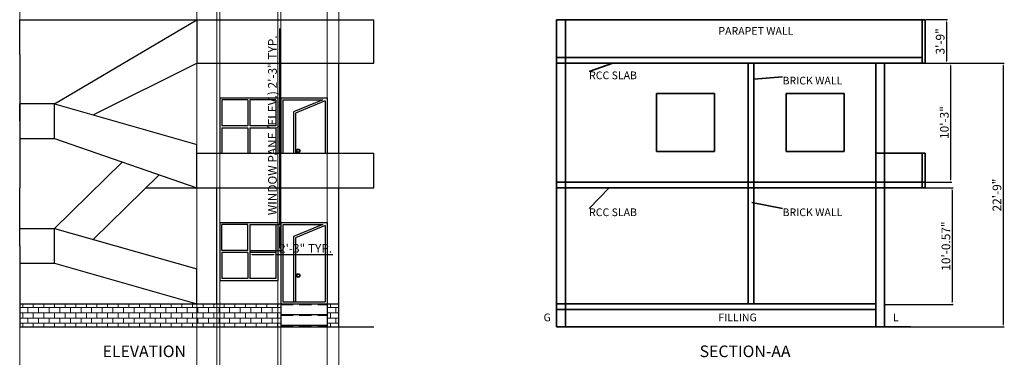
# Model space of a CAD drawing. Units: inches. Extents: x 57 to 1276, y 38 to 1417.
# Tile 2 of 2: x 162 to 1180, y 1068 to 1417. Entities that reach past the tile are written whole.
import ezdxf

# ---------------------------------------------------------------- set-up
doc = ezdxf.new("R2010")
doc.units = ezdxf.units.IN
doc.linetypes.add('DASHED', pattern=[19.05, 12.7, -6.35])
for name, color, linetype, lineweight in [('A-ANNO-DIMS', 2, 'Continuous', 18), ('A-ANNO-TEXT', 7, 'Continuous', 18), ('A-CONS', 9, 'Continuous', 13), ('A-ELEV', 7, 'Continuous', 25), ('A-ELEV-OVHD', 8, 'DASHED', 18), ('A-ELEV-PATT', 8, 'Continuous', 13), ('A-SECT', 7, 'Continuous', 35)]:
    doc.layers.add(name, color=color, linetype=linetype, lineweight=lineweight)
doc.styles.get("Standard").update_dxf_attribs({"font": 'arial.ttf'})
doc.dimstyles.new('ISO-25', dxfattribs={"dimtxt": 9, "dimasz": 2.5, "dimexe": 1.25, "dimexo": 0.625, "dimtad": 1, "dimlunit": 3, "dimtxsty": 'Standard', "dimcen": 2.5, "dimadec": 0, "dimazin": 0, "dimtfac": 1, "dimtmove": 0, "dimatfit": 3, "dimfxl": 1, "dimarcsym": 0})

# ---------------------------------------------------------------- blocks, each defined once
blk = doc.blocks.new('*D16')
at = {"layer": 'A-ANNO-DIMS', "color": 0, "lineweight": -2, "transparency": 16777216}
for p, q in [((1098.3, 1417), (1120.9, 1417)), ((1119.6, 1414.5), (1119.6, 1374.5)), ((1098.3, 1372), (1120.9, 1372))]:
    blk.add_line(p, q, dxfattribs=at)
at = {"layer": 'A-ANNO-DIMS', "color": 0, "transparency": 16777216}
for points in [[(1119.2, 1414.5), (1120, 1414.5), (1119.6, 1417)], [(1119.2, 1374.5), (1120, 1374.5), (1119.6, 1372)]]:
    blk.add_solid(points, dxfattribs=at)
at = {"layer": 'Defpoints', "color": 0, "transparency": 16777216}
for p in [(1097.7, 1417), (1097.7, 1372), (1119.6, 1372)]:
    blk.add_point(p, dxfattribs=at)
at = {"layer": 'A-ANNO-DIMS', "color": 0, "transparency": 16777216, "insert": (1114.4, 1394.5), "char_height": 9, "attachment_point": 5, "rotation": 90}
blk.add_mtext('3\'-9"', dxfattribs=at)
blk = doc.blocks.new('*D17')
at = {"layer": 'A-ANNO-DIMS', "color": 0, "lineweight": -2, "transparency": 16777216}
for p, q in [((1056.3, 1372), (1179.5, 1372)), ((1178.3, 1369.5), (1178.3, 1101.5)), ((1056.3, 1099), (1179.5, 1099))]:
    blk.add_line(p, q, dxfattribs=at)
at = {"layer": 'A-ANNO-DIMS', "color": 0, "transparency": 16777216}
for points in [[(1177.9, 1369.5), (1178.7, 1369.5), (1178.3, 1372)], [(1177.9, 1101.5), (1178.7, 1101.5), (1178.3, 1099)]]:
    blk.add_solid(points, dxfattribs=at)
at = {"layer": 'Defpoints', "color": 0, "transparency": 16777216}
for p in [(1055.7, 1372), (1055.7, 1099), (1178.3, 1099)]:
    blk.add_point(p, dxfattribs=at)
at = {"layer": 'A-ANNO-DIMS', "color": 0, "transparency": 16777216, "insert": (1173.1, 1235.5), "char_height": 9, "attachment_point": 5, "rotation": 90}
blk.add_mtext('22\'-9"', dxfattribs=at)
blk = doc.blocks.new('*D18')
at = {"layer": 'A-ANNO-DIMS', "color": 0, "lineweight": -2, "transparency": 16777216}
for p, q in [((1056.3, 1372), (1125.2, 1372)), ((1123.9, 1369.5), (1123.9, 1251.5)), ((1056.3, 1249), (1125.2, 1249))]:
    blk.add_line(p, q, dxfattribs=at)
at = {"layer": 'A-ANNO-DIMS', "color": 0, "transparency": 16777216}
for points in [[(1123.5, 1369.5), (1124.3, 1369.5), (1123.9, 1372)], [(1123.5, 1251.5), (1124.3, 1251.5), (1123.9, 1249)]]:
    blk.add_solid(points, dxfattribs=at)
at = {"layer": 'Defpoints', "color": 0, "transparency": 16777216}
for p in [(1055.7, 1372), (1055.7, 1249), (1123.9, 1249)]:
    blk.add_point(p, dxfattribs=at)
at = {"layer": 'A-ANNO-DIMS', "color": 0, "transparency": 16777216, "insert": (1118.7, 1310.5), "char_height": 9, "attachment_point": 5, "rotation": 90}
blk.add_mtext('10\'-3"', dxfattribs=at)
blk = doc.blocks.new('*D19')
at = {"layer": 'A-ANNO-DIMS', "color": 0, "lineweight": -2, "transparency": 16777216}
for p, q in [((1056.3, 1243), (1126.7, 1243)), ((1125.5, 1240.5), (1125.5, 1124.9)), ((1056.3, 1122.4), (1126.7, 1122.4))]:
    blk.add_line(p, q, dxfattribs=at)
at = {"layer": 'A-ANNO-DIMS', "color": 0, "transparency": 16777216}
for points in [[(1125.1, 1240.5), (1125.9, 1240.5), (1125.5, 1243)], [(1125.1, 1124.9), (1125.9, 1124.9), (1125.5, 1122.4)]]:
    blk.add_solid(points, dxfattribs=at)
at = {"layer": 'Defpoints', "color": 0, "transparency": 16777216}
for p in [(1055.7, 1243), (1055.7, 1122.4), (1125.5, 1122.4)]:
    blk.add_point(p, dxfattribs=at)
at = {"layer": 'A-ANNO-DIMS', "color": 0, "transparency": 16777216, "insert": (1120.3, 1182.7), "char_height": 9, "attachment_point": 5, "rotation": 90}
blk.add_mtext('10\'-0.57"', dxfattribs=at)
blk = doc.blocks.new('WIN-ELEV-PANE')
for p, q in [((0, 27), (0, 0)), ((0, 27), (27, 27)), ((27, 27), (27, 0)), ((0, 0), (27, 0))]:
    blk.add_line(p, q)
blk = doc.blocks.new('*D33')
at = {"layer": 'A-ANNO-DIMS', "color": 0, "lineweight": -2, "transparency": 16777216}
for p, q in [((430.6, 1205), (430.6, 1407.9)), ((427.1, 1205), (431.8, 1205)), ((430.6, 1180.5), (430.6, 1202.5)), ((427.1, 1178), (431.8, 1178))]:
    blk.add_line(p, q, dxfattribs=at)
at = {"layer": 'A-ANNO-DIMS', "color": 0, "transparency": 16777216}
for points in [[(430.2, 1202.5), (431, 1202.5), (430.6, 1205)], [(430.2, 1180.5), (431, 1180.5), (430.6, 1178)]]:
    blk.add_solid(points, dxfattribs=at)
at = {"layer": 'Defpoints', "color": 0, "transparency": 16777216}
for p in [(426.5, 1205), (430.6, 1205), (426.5, 1178)]:
    blk.add_point(p, dxfattribs=at)
at = {"layer": 'A-ANNO-DIMS', "color": 0, "transparency": 16777216, "insert": (424, 1307.7), "char_height": 9, "attachment_point": 5, "rotation": 90}
blk.add_mtext('WINDOW PANE (ELEV.) 2\'-3" TYP.', dxfattribs=at)
blk = doc.blocks.new('*D34')
at = {"layer": 'A-ANNO-DIMS', "color": 0, "lineweight": -2, "transparency": 16777216}
for p, q in [((399.5, 1177.4), (399.5, 1172.7)), ((402, 1173.9), (424, 1173.9)), ((426.5, 1177.4), (426.5, 1172.7)), ((426.5, 1173.9), (485.3, 1173.9))]:
    blk.add_line(p, q, dxfattribs=at)
at = {"layer": 'A-ANNO-DIMS', "color": 0, "transparency": 16777216}
for points in [[(402, 1174.4), (402, 1173.5), (399.5, 1173.9)], [(424, 1174.4), (424, 1173.5), (426.5, 1173.9)]]:
    blk.add_solid(points, dxfattribs=at)
at = {"layer": 'Defpoints', "color": 0, "transparency": 16777216}
for p in [(399.5, 1178), (426.5, 1178), (426.5, 1173.9)]:
    blk.add_point(p, dxfattribs=at)
at = {"layer": 'A-ANNO-DIMS', "color": 0, "transparency": 16777216, "insert": (457.1, 1179.2), "char_height": 9, "attachment_point": 5}
blk.add_mtext('2\'-3" TYP.', dxfattribs=at)

msp = doc.modelspace()

# ---------------------------------------------------------------- hatches: boundary and pattern name
at = {"layer": 'A-ELEV-PATT'}
h = msp.add_hatch(dxfattribs=at)
h.set_pattern_fill('AR-B816', color=256, scale=0.027)
h.paths.add_polyline_path([(431.517, 1122.986), (161.517, 1122.986), (161.517, 1098.986), (431.517, 1098.986)])
h.paths.add_polyline_path([(491.517, 1122.986), (479.517, 1122.986), (479.517, 1098.986), (491.517, 1098.986)])

# ---------------------------------------------------------------- linework, layer by layer
at = {"layer": 'A-CONS'}
for p in [(161.517, 877.429), (161.517, 175.429), (344.517, 175.429), (365.517, 304.429), (368.517, 364.429), (428.517, 364.429), (431.517, 368.029), (479.517, 364.429), (491.517, 364.429)]:
    msp.add_xline(p, (0, 1), dxfattribs=at)
at = {"layer": 'A-ELEV'}
for p, q in [((161.517, 1416.986), (527.517, 1416.986)), ((161.517, 1380.986), (161.517, 1416.986)), ((197.517, 1329.986), (344.517, 1416.986)), ((344.517, 1416.986), (344.517, 1371.986)), ((527.517, 1371.986), (527.517, 1416.986)), ((161.517, 1380.986), (161.517, 1242.986)), ((237.345, 1318.607), (344.517, 1371.986)), ((344.517, 1371.986), (527.517, 1371.986)), ((491.517, 1278.986), (491.517, 1371.986)), ((368.517, 1335.986), (428.517, 1335.986)), ((368.517, 1335.986), (368.517, 1278.986)), ((428.517, 1335.986), (428.517, 1278.986)), ((431.517, 1335.986), (479.517, 1335.986)), ((431.517, 1335.986), (431.517, 1278.986)), ((433.517, 1333.986), (474.867, 1333.986)), ((433.517, 1333.986), (433.517, 1278.986)), ((474.867, 1333.986), (444.517, 1321.619)), ((479.517, 1335.986), (479.517, 1278.986)), ((161.517, 1311.986), (161.517, 1329.986)), ((197.517, 1329.986), (161.517, 1329.986)), ((197.517, 1329.986), (344.517, 1287.986)), ((197.517, 1293.986), (197.517, 1329.986)), ((477.517, 1332.906), (446.517, 1320.275)), ((477.517, 1332.906), (477.517, 1278.986)), ((444.517, 1321.619), (444.517, 1278.986)), ((446.517, 1320.275), (446.517, 1278.986)), ((370.517, 1304.986), (370.517, 1278.986)), ((370.517, 1304.986), (397.517, 1304.986)), ((397.517, 1304.986), (397.517, 1278.986)), ((399.517, 1304.986), (399.517, 1278.986)), ((399.517, 1304.986), (426.517, 1304.986)), ((426.517, 1304.986), (426.517, 1278.986)), ((161.517, 1293.986), (197.517, 1293.986)), ((197.517, 1293.986), (344.517, 1242.986)), ((344.517, 1242.986), (344.517, 1287.986)), ((344.517, 1278.986), (527.517, 1278.986)), ((527.517, 1242.986), (527.517, 1278.986)), ((197.517, 1200.986), (267.625, 1269.663)), ((237.345, 1189.607), (305.615, 1256.483)), ((161.517, 1182.986), (161.517, 1242.986)), ((291.837, 1242.986), (527.517, 1242.986)), ((365.517, 1122.986), (365.517, 1242.986)), ((491.517, 1098.986), (491.517, 1242.986)), ((368.517, 1206.986), (428.517, 1206.986)), ((368.517, 1206.986), (368.517, 1146.986)), ((428.517, 1206.986), (428.517, 1146.986)), ((431.517, 1206.986), (431.517, 1122.986)), ((431.517, 1206.986), (479.517, 1206.986)), ((433.517, 1204.986), (474.867, 1204.986)), ((433.517, 1204.986), (433.517, 1124.986)), ((474.867, 1204.986), (444.517, 1192.619)), ((477.517, 1203.906), (446.517, 1191.275)), ((477.517, 1203.906), (477.517, 1124.986)), ((479.517, 1206.986), (479.517, 1122.986)), ((161.517, 1200.986), (197.517, 1200.986)), ((197.517, 1200.986), (344.517, 1158.986)), ((197.517, 1164.986), (197.517, 1200.986)), ((444.517, 1192.619), (444.517, 1124.986)), ((446.517, 1191.275), (446.517, 1124.986)), ((161.517, 1182.986), (161.517, 1098.986)), ((161.517, 1164.986), (197.517, 1164.986)), ((197.517, 1164.986), (344.517, 1122.986)), ((344.517, 1122.986), (344.517, 1158.986)), ((368.517, 1146.986), (428.517, 1146.986)), ((161.517, 1122.986), (491.517, 1122.986)), ((431.517, 1122.986), (431.517, 1098.986)), ((433.517, 1124.986), (477.517, 1124.986)), ((479.517, 1122.986), (479.517, 1098.986)), ((431.517, 1111.986), (479.517, 1111.986)), ((431.517, 1100.986), (479.517, 1100.986)), ((161.517, 1098.986), (527.517, 1098.986))]:
    msp.add_line(p, q, dxfattribs=at)
for centre, radius in [((449.515, 1281.211), 1.951), ((449.515, 1281.211), 1.351), ((449.515, 1152.211), 1.951), ((449.515, 1152.211), 1.351)]:
    msp.add_circle(centre, radius, dxfattribs=at)
at = {"layer": 'A-ELEV-OVHD'}
for p, q in [((431.517, 1121.986), (479.517, 1121.986)), ((431.517, 1110.986), (479.517, 1110.986)), ((431.517, 1099.986), (479.517, 1099.986))]:
    msp.add_line(p, q, dxfattribs=at)
at = {"layer": 'A-SECT'}
for p, q in [((716.695, 1416.986), (1097.695, 1416.986)), ((716.695, 1098.986), (716.695, 1416.986)), ((725.695, 1098.986), (725.695, 1416.986)), ((1094.695, 1371.986), (1094.695, 1416.986)), ((1097.695, 1371.986), (1097.695, 1416.986)), ((716.695, 1377.986), (1094.695, 1377.986)), ((716.695, 1371.986), (1097.695, 1371.986)), ((774.627, 1371.986), (750.228, 1363.36)), ((914.695, 1122.986), (914.695, 1371.986)), ((920.695, 1122.986), (920.695, 1371.986)), ((1046.695, 1098.986), (1046.695, 1371.986)), ((1055.695, 1098.986), (1055.695, 1371.986)), ((920.695, 1355.534), (950.238, 1357.923)), ((819.768, 1340.511), (879.768, 1340.511)), ((819.768, 1340.511), (819.768, 1280.511)), ((879.768, 1340.511), (879.768, 1280.511)), ((954.135, 1340.511), (1014.135, 1340.511)), ((954.135, 1340.511), (954.135, 1280.511)), ((1014.135, 1340.511), (1014.135, 1280.511)), ((819.768, 1280.511), (879.768, 1280.511)), ((954.135, 1280.511), (1014.135, 1280.511)), ((1046.695, 1278.986), (1097.695, 1278.986)), ((1094.695, 1242.986), (1094.695, 1278.986)), ((1097.695, 1242.986), (1097.695, 1278.986)), ((716.695, 1248.986), (1097.695, 1248.986)), ((716.695, 1242.986), (1097.695, 1242.986)), ((771.016, 1242.986), (750.228, 1221.67)), ((918.39, 1227.916), (950.238, 1221.67)), ((716.695, 1122.986), (1046.695, 1122.986)), ((716.695, 1116.986), (1046.695, 1116.986)), ((716.695, 1098.986), (1082.695, 1098.986))]:
    msp.add_line(p, q, dxfattribs=at)

# ---------------------------------------------------------------- block references
at = {"layer": 'A-ELEV'}
for p, rotation in [((370.517, 1333.986), 270), ((399.517, 1333.986), 270), ((397.517, 1204.987), 180), ((370.517, 1175.986), 270), ((399.517, 1175.986), 270)]:
    msp.add_blockref('WIN-ELEV-PANE', p, dxfattribs=dict(at, rotation=rotation))
msp.add_blockref('WIN-ELEV-PANE', (399.517, 1177.986), dxfattribs=at)

# ---------------------------------------------------------------- texts
at = {"layer": 'A-ANNO-TEXT', "attachment_point": 1}
for s, width, insert, char_height in [('PARAPET WALL', 90.54643, (883.943, 1409.32), 8), ('RCC SLAB', 60.5935, (750.228, 1363.36), 8), ('BRICK WALL', 69.50041, (950.238, 1357.923), 8), ('RCC SLAB', 60.5935, (750.228, 1221.67), 8), ('BRICK WALL', 69.50041, (950.238, 1221.67), 8), ('G', 8.01484, (703.151, 1112.877), 8), ('FILLING', 60.5935, (883.943, 1112.877), 8), ('L', 8.01484, (1064.432, 1112.877), 8), ('ELEVATION', 97.694, (247.312, 1079.794), 12), ('SECTION-AA', 109.11559, (864.545, 1079.794), 12)]:
    msp.add_mtext_dynamic_manual_height_columns(s, width=width, gutter_width=12.5, heights=[0], dxfattribs=dict(at, insert=insert, char_height=char_height))

# ---------------------------------------------------------------- dimensions: what is measured, and where the dimension line sits
at = {"layer": 'A-ANNO-DIMS'}
for base, p1, p2, picture, middle in [((1119.603, 1371.986), (1097.695, 1416.986), (1097.695, 1371.986), '*D16', (1114.38, 1394.486)), ((1178.287, 1098.986), (1055.695, 1371.986), (1055.695, 1098.986), '*D17', (1173.067, 1235.486)), ((1123.923, 1248.986), (1055.695, 1371.986), (1055.695, 1248.986), '*D18', (1118.7, 1310.486)), ((1125.4978, 1122.4212), (1055.695, 1242.9863), (1055.695, 1122.4212), '*D19', (1120.2777, 1182.7037))]:
    dim = msp.add_linear_dim(base=base, p1=p1, p2=p2, angle=90, dimstyle='ISO-25', override={"dimclrd": 0, "dimclre": 0, "dimclrt": 0}, dxfattribs=at)
    dim.commit()
    dim.dimension.update_dxf_attribs({"geometry": picture, "text_midpoint": middle})
dim = msp.add_linear_dim(base=(430.567, 1204.986), p1=(426.517, 1177.986), p2=(426.517, 1204.986), angle=90, text='WINDOW PANE (ELEV.) <> TYP.', dimstyle='ISO-25', override={"dimdec": 1, "dimrnd": 0, "dimzin": 1, "dimlunit": 4, "dimfrac": 2}, dxfattribs=at)
dim.commit()
dim.dimension.update_dxf_attribs({"geometry": '*D33', "text_midpoint": (424.039, 1307.676)})
dim = msp.add_linear_dim(base=(426.517, 1173.936), p1=(399.517, 1177.986), p2=(426.517, 1177.986), text='<> TYP.', dimstyle='ISO-25', override={"dimdec": 1, "dimrnd": 0, "dimzin": 1, "dimlunit": 4, "dimfrac": 2}, dxfattribs=at)
dim.commit()
dim.dimension.update_dxf_attribs({"geometry": '*D34', "text_midpoint": (457.148, 1179.159)})

doc.saveas('drawing.dxf')
